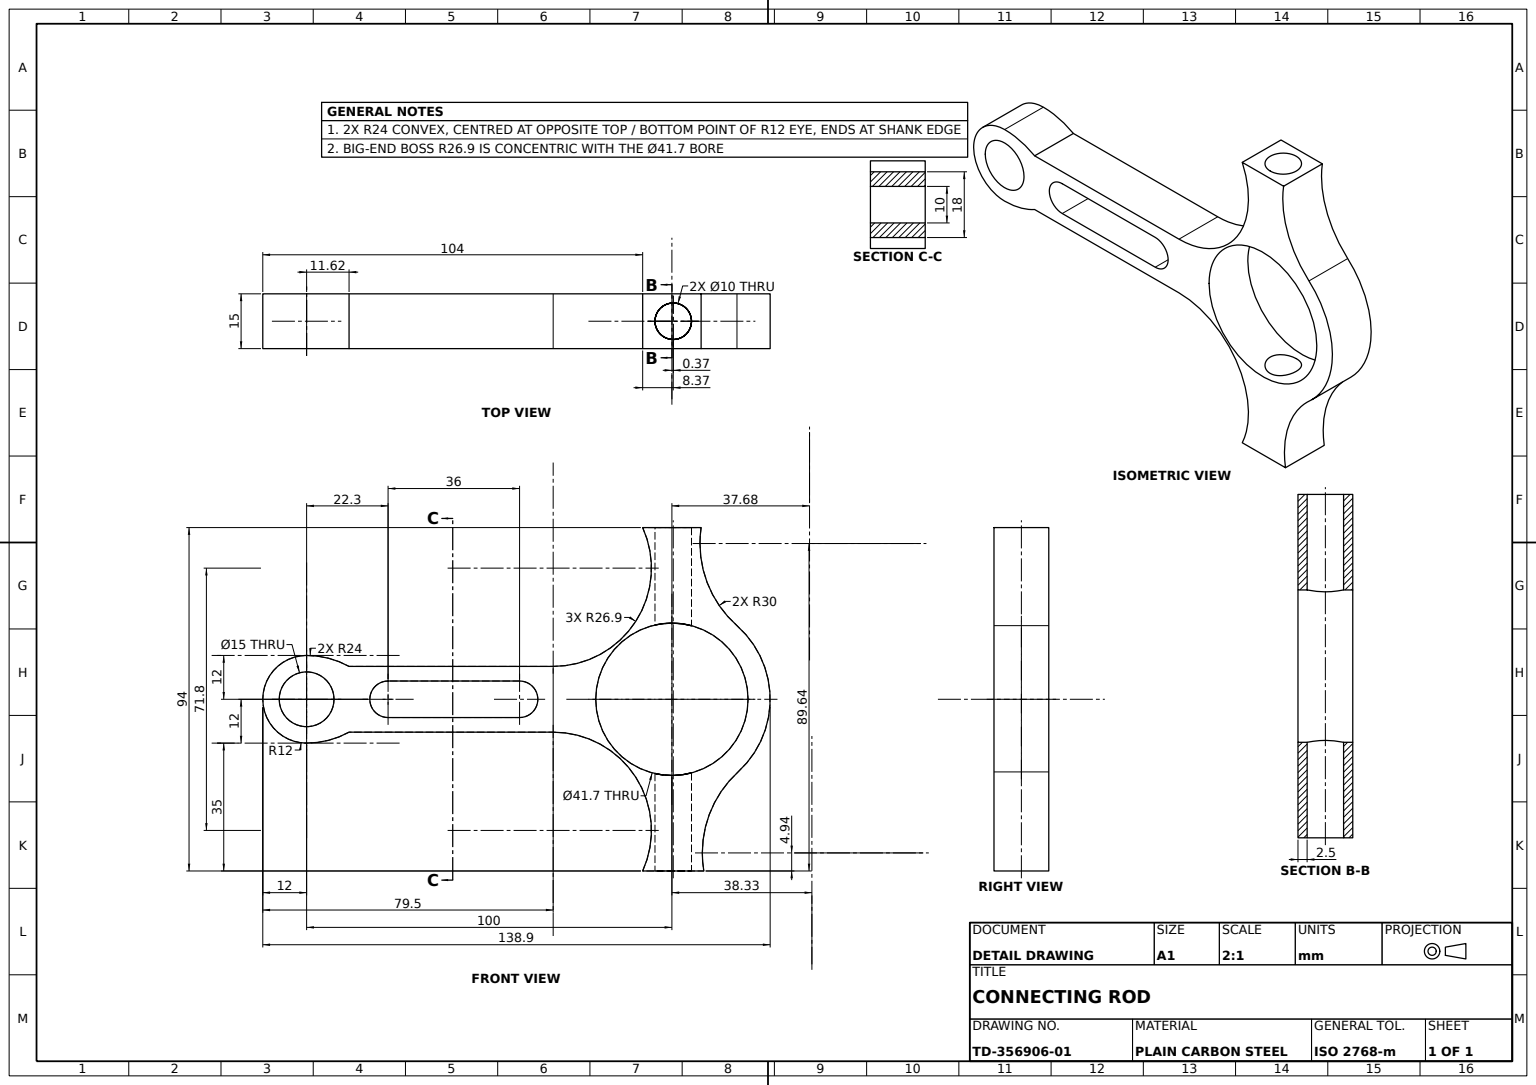
SolidWorks part; units mm, degrees
material "Plain Carbon Steel"
ref_plane "Front Plane" through (0, 0, 0) normal (0, 0, 1) x (1, 0, 0)
ref_plane "Top Plane" through (0, 0, 0) normal (0, 1, 0) x (1, 0, 0)
ref_plane "Right Plane" through (0, 0, 0) normal (1, 0, 0) x (0, 0, -1)
sketch "Link Profile Sketch" plane through (0, 0, 0) normal (0, 0, 1) x (1, 0, 0)
  line L0 (0, 0) -> (100, 0) construction
  line L1 (100, 0) -> (100, 47) construction
  line L2 (100, 0) -> (100, -47) construction
  line L3 (100, 47) -> (92, 47)
  line L4 (100, 47) -> (108, 47)
  line L5 (100, -47) -> (92, -47)
  line L6 (100, -47) -> (108.7366, -47)
  line L7 (11.619, -9) -> (67.4969, -9)
  line L8 (11.619, 9) -> (67.4969, 9)
  line L9 (22.3, -5) -> (58.3, -5)
  line L10 (0, 9) -> (100, 9) construction
  line L11 (0, -9) -> (100, -9) construction
  line L12 (22.3, 5) -> (58.3, 5)
  line L13 (7.5, 0) -> (73.1, 0) construction
  line L14 (0, 5) -> (100, 5) construction
  line L15 (0, -5) -> (100, -5) construction
  line L16 (40.3, 0) -> (22.3, 0) construction
  line L17 (40.3, 0) -> (58.3, 0) construction
  circle A0 centre (0, 0) radius 7.5
  arc A1 (0, 12) -> (0, -12) centre (0, 0) ccw
  circle A2 centre (100, 0) radius 20.85
  arc A3 (118.1191, -19.8823) -> (117.8139, 20.1562) centre (100, 0) ccw
  arc A4 (108, 47) -> (117.8139, 20.1562) centre (137.6808, 42.6353) ccw
  arc A5 (108.7366, -47) -> (118.1191, -19.8823) centre (138.3264, -42.0559) cw
  arc A6 (0, 12) -> (11.619, 9) centre (0, -12) cw
  arc A7 (0, -12) -> (11.619, -9) centre (0, 12) ccw
  arc A8 (22.3, 5) -> (22.3, -5) centre (22.3, 0) ccw
  arc A9 (58.3, -5) -> (58.3, 5) centre (58.3, 0) ccw
  arc A10 (92, 47) -> (67.4969, 9) centre (67.4969, 35.9) cw
  arc A12 (92, -47) -> (67.4969, -9) centre (67.4969, -35.9) ccw
  dimension "D1" = 41.7
  dimension "D2" = 15
  dimension "D3" = 24
  dimension "D4" = 53.8
  dimension "D7" = 30
  dimension "D8" = 47
  dimension "D11" = 5
  dimension "D12" = 5
  dimension "D15" = 26.9
  dimension "D16" = 16
  dimension "D18" = 30
  dimension "D19" = 26.9
  dimension "D5" = 100
  dimension "D6" = 47
  dimension "D13" = 11.619
  dimension "D14" = 11.619
  dimension "D17" = 16.7366
  dimension "D20" = 65.6
  dimension "D21" = 36
  dimension "D9" = 5
  dimension "D10" = 5
extrude "Link Body 15mm" add sketch "Link Profile Sketch" along normal blind 15
sketch "Bolt Hole Sketch" plane through (0, -47, 0) normal (0, -1, 0) x (1, 0, 0)
  line L0 (108.7366, 15) -> (108.7366, 0) construction
  line L1 (92, 0) -> (108.7366, 0) construction
  circle A0 centre (100.3683, 7.5) radius 5
  dimension "D1" = 10
  dimension "D2" = 8.3683
  dimension "D3" = 7.5
extrude "Bolt Hole Ø10" cut sketch "Bolt Hole Sketch" against normal through all
